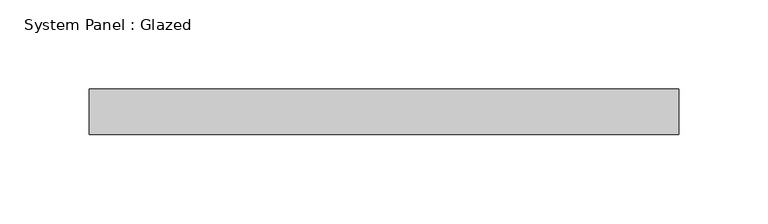
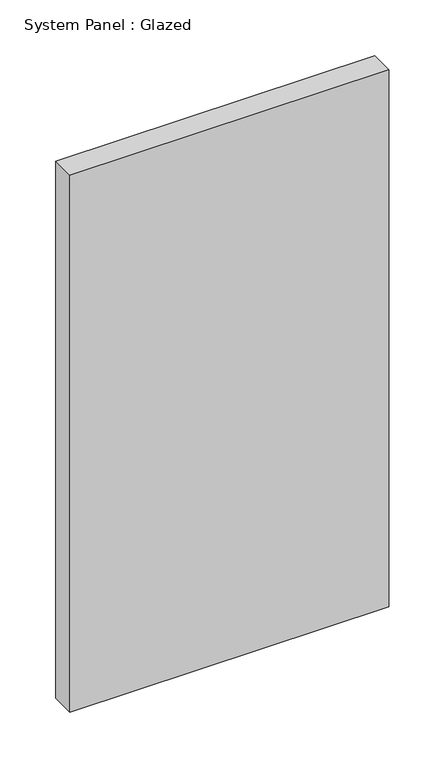
"""IFC4 building model written with IfcOpenShell, lengths in millimetres: plate geometry, System Panel : Glazed."""

from ifc_helpers import new_model, si_unit, origin, origin_with_axes, place, context, project, spatial, polyline, outline, extrude, source, transform, mapped, element, save


def system_panel_glazed_09b5f287(model_context):
    return source(origin(), model_context, "Body", "SweptSolid", [
        extrude(outline(polyline([(165.1, 19.05), (-165.1, 19.05), (-165.1, 44.45), (165.1, 44.45), (165.1, 19.05)])), origin_with_axes(), (0.0, 0.0, 1.0), 587.6147026),
    ])


if __name__ == "__main__":
    model = new_model("IFC4")
    model_context = context("Model", 3, world=origin())
    ifc_project = project(units=[si_unit("LENGTHUNIT", "METRE", prefix="MILLI")], contexts=[model_context])
    site = spatial("IfcSite", under=ifc_project)
    building = spatial("IfcBuilding", under=site)
    placement = place(None, origin())
    system_panel_glazed_shape = system_panel_glazed_09b5f287(model_context)
    element("IfcPlate", 1, ObjectType="System Panel : Glazed", at=placement, inside=building, context=model_context, shape_type="MappedRepresentation", body=[
        mapped(system_panel_glazed_shape, transform((0.0, 0.0, 0.0), x_axis=(1.0, 0.0, 0.0), y_axis=(0.0, 1.0, 0.0), z_axis=(0.0, 0.0, 1.0))),
    ])
    save(model, "model.ifc")

# Revit data of these elements
# Type "System Panel : Glazed"
#   Construction Type Id = "GSP4R"
#   Analytic Construction = "1/8 in Pilkington single glazing"
#   Visual Light Transmittance = 0.9
#   Solar Heat Gain Coefficient = 0.86
#   Heat Transfer Coefficient (U) = 1.18115 BTU/(h·ft²·°F)
#   Define Thermal Properties by = 1
# Element 1 (IfcPlate, "System Panel : Glazed")
#   Materials on its faces: "Glass"
# Materials
#   "Glass": class "Glass", colour RGB 0 128 192, transparency 0.75, Description = "Soda Lime Glass", Cost = 0
